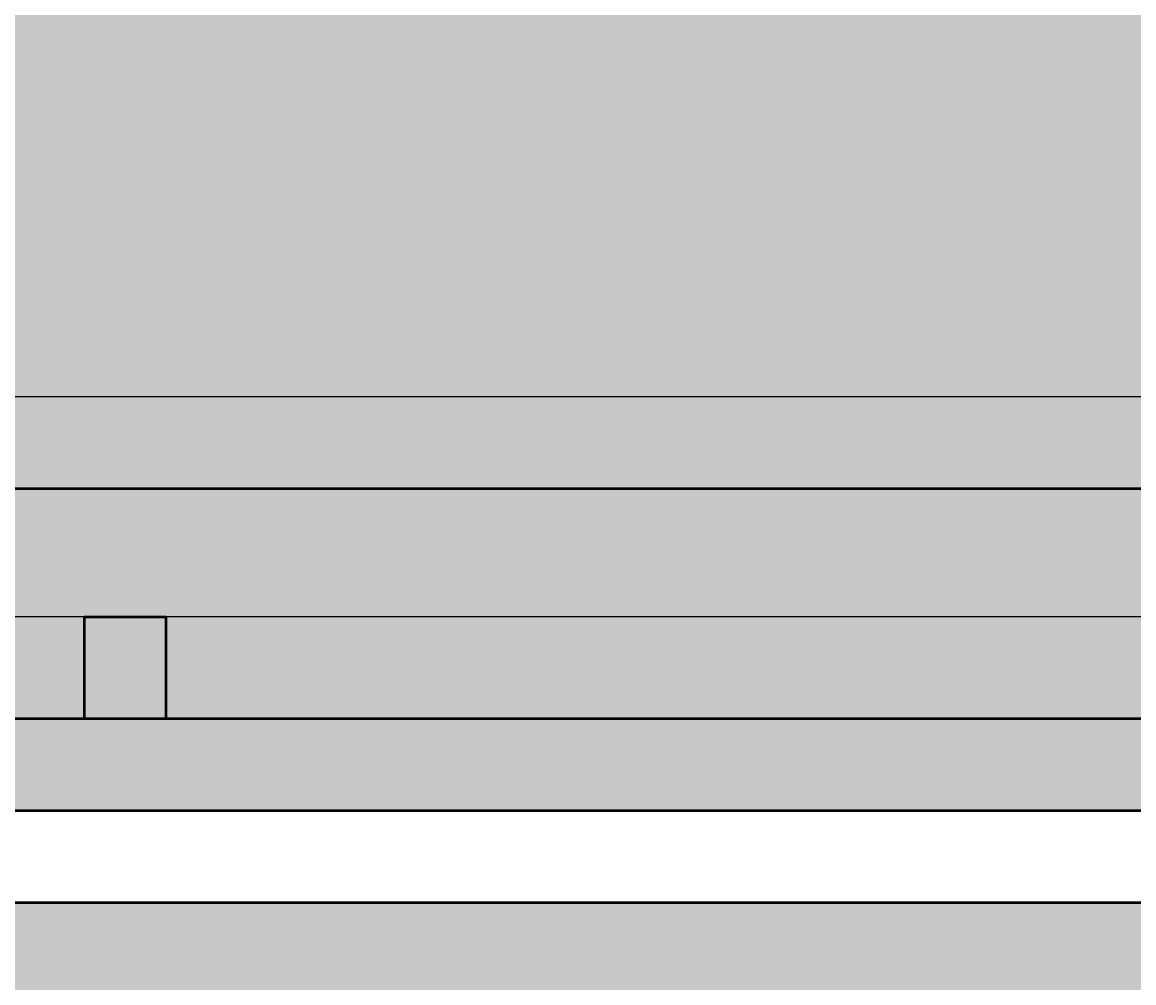
# Model space of a CAD drawing. Units: inches. Extents: x -12 to 334, y -10 to 186.
# Tile 40 of 77: x 128 to 152, y 90 to 111. Entities that reach past the tile are written whole.
import ezdxf
from ezdxf import colors
from ezdxf.entities.mleader import LeaderData, LeaderLine
from ezdxf.math import Vec2, Vec3

# ---------------------------------------------------------------- set-up
doc = ezdxf.new("R2010")
doc.units = ezdxf.units.IN
doc.header["$MEASUREMENT"] = 0
for name, color, linetype, lineweight in [('M-ANNO-TEXT', 3, 'Continuous', 25), ('M-DIMS', 2, 'Continuous', 18), ('M-EQPM', 7, 'Continuous', 50), ('M-EQPM-PATT', 8, 'Continuous', 18)]:
    doc.layers.add(name, color=color, linetype=linetype, lineweight=lineweight)
doc.styles.get("Standard").update_dxf_attribs({"font": 'arial.ttf'})
doc.dimstyles.get("Standard").update_dxf_attribs({"dimtxt": 0.18, "dimasz": 0.18, "dimexe": 0.18, "dimexo": 0.0625, "dimgap": 0.09, "dimtad": 0, "dimtih": 1, "dimtoh": 1, "dimdec": 4, "dimzin": 0, "dimdsep": 46, "dimtxsty": 'Standard', "dimcen": 0.09, "dimadec": 0, "dimazin": 0, "dimtfac": 1, "dimtdec": 4, "dimtofl": 0, "dimtmove": 0, "dimatfit": 3, "dimfxl": 1, "dimtolj": 1, "dimtzin": 0, "dimarcsym": 0})

# ---------------------------------------------------------------- blocks, each defined once
blk = doc.blocks.new('*D1')
at = {"layer": 'Defpoints', "color": 0, "transparency": 16777216}
for p in [(281.426, 91.899), (3.376, 80.692), (281.426, 14.304)]:
    blk.add_point(p, dxfattribs=at)
at = {"layer": 'M-DIMS', "color": 0, "lineweight": -2, "transparency": 16777216}
for p, q in [((281.426, 91.836), (281.426, 14.124)), ((3.376, 80.629), (3.376, 14.124)), ((3.556, 14.304), (141.935, 14.304)), ((281.246, 14.304), (142.867, 14.304))]:
    blk.add_line(p, q, dxfattribs=at)
at = {"layer": 'M-DIMS', "color": 0, "transparency": 16777216}
for points in [[(3.556, 14.334), (3.556, 14.274), (3.376, 14.304)], [(281.246, 14.334), (281.246, 14.274), (281.426, 14.304)]]:
    blk.add_solid(points, dxfattribs=at)
at = {"layer": 'M-DIMS', "color": 0, "transparency": 16777216, "insert": (142.401, 14.304), "char_height": 0.18, "attachment_point": 5}
blk.add_mtext('\\A1;278.05', dxfattribs=at)
blk = doc.blocks.new('*D17')
at = {"layer": 'Defpoints', "color": 0, "transparency": 16777216}
for p in [(106.177, 102.896), (105.892, 56.321), (295.976, 56.321)]:
    blk.add_point(p, dxfattribs=at)
at = {"layer": 'M-DIMS', "color": 0, "lineweight": -2, "transparency": 16777216}
for p, q in [((106.24, 102.896), (296.156, 102.896)), ((295.976, 102.716), (295.976, 79.79)), ((295.976, 56.501), (295.976, 79.426)), ((105.954, 56.321), (296.156, 56.321))]:
    blk.add_line(p, q, dxfattribs=at)
at = {"layer": 'M-DIMS', "color": 0, "transparency": 16777216}
for points in [[(295.946, 102.716), (296.006, 102.716), (295.976, 102.896)], [(295.946, 56.501), (296.006, 56.501), (295.976, 56.321)]]:
    blk.add_solid(points, dxfattribs=at)
at = {"layer": 'M-DIMS', "color": 0, "transparency": 16777216, "insert": (295.976, 79.608), "char_height": 0.18, "attachment_point": 5}
blk.add_mtext('\\A1;46.575', dxfattribs=at)
blk = doc.blocks.new('*D35')
at = {"layer": 'Defpoints', "color": 0, "transparency": 16777216}
for p in [(216.428, 98.108), (-11.174, 61.105), (216.428, 61.105)]:
    blk.add_point(p, dxfattribs=at)
at = {"layer": 'M-DIMS', "color": 0, "lineweight": -2, "transparency": 16777216}
for p, q in [((216.365, 98.108), (-11.354, 98.108)), ((-11.174, 97.928), (-11.174, 79.788)), ((-11.174, 61.285), (-11.174, 79.424)), ((216.365, 61.105), (-11.354, 61.105))]:
    blk.add_line(p, q, dxfattribs=at)
at = {"layer": 'M-DIMS', "color": 0, "transparency": 16777216}
for points in [[(-11.204, 97.928), (-11.144, 97.928), (-11.174, 98.108)], [(-11.204, 61.285), (-11.144, 61.285), (-11.174, 61.105)]]:
    blk.add_solid(points, dxfattribs=at)
at = {"layer": 'M-DIMS', "color": 0, "transparency": 16777216, "insert": (-11.174, 79.606), "char_height": 0.18, "attachment_point": 5}
blk.add_mtext('\\A1;37', dxfattribs=at)

msp = doc.modelspace()

# ---------------------------------------------------------------- hatches: boundary and pattern name
at = {"layer": 'M-EQPM-PATT', "transparency": 33554556}
h = msp.add_hatch(color=256, dxfattribs=at)
h.set_gradient(color1=(248, 206, 179), color2=(248, 206, 179), tint=1)
h.paths.add_polyline_path([(179.7818, 136.8871), (126.9567, 136.8871), (106.1771, 100.8958), (171.5458, 100.8958)])
h.paths.add_polyline_path([(268.3808, 136.9435), (214.0166, 136.9435), (214.0166, 154.8345), (196.3421, 154.8345), (196.3421, 136.8871), (179.7818, 136.8871), (171.5458, 100.8958), (231.7758, 100.8958, -0.4142136), (251.9801, 80.6915), (279.7263, 80.6915, 0.1631825)])
at = {"layer": 'M-EQPM-PATT'}
h = msp.add_hatch(color=256, dxfattribs=at)
h.set_gradient(color1=(205, 32, 39), color2=(205, 32, 39), tint=1)
h.paths.add_polyline_path([(64.5, 80.754), (64.5, 89.8963), (226.6083, 89.8963, -1), (226.6083, 69.6117), (64.5, 69.6117), (64.5, 78.754), (4.4744, 78.754, 0.384914), (23.5807, 61.4872), (37.1002, 61.4872), (37.1002, 33.6752), (53.1002, 33.6752), (53.1002, 61.4872), (64.5, 61.4872), (64.5, 63.6117), (226.6083, 63.6117, 1), (226.6083, 95.8963), (64.5, 95.8963), (64.5, 99.8958), (53.1002, 99.8958), (53.1002, 127.7078), (37.1002, 127.7078), (37.1002, 99.8958), (23.5807, 99.8958, 0.4132606), (4.3766, 80.754)])
h.paths.add_polyline_path([(64.5, 91.8963), (64.5, 93.8963), (226.6083, 93.8963, -1), (226.6083, 65.6117), (64.5, 65.6117), (64.5, 67.6117), (226.6083, 67.6117, 1), (226.6083, 91.8963)], flags=16)
h = msp.add_hatch(color=256, dxfattribs=at)
h.set_gradient(color1=(99, 100, 102), color2=(99, 100, 102), tint=1)
h.paths.add_polyline_path([(72.9244, 95.8963), (75.9244, 95.8963), (75.9244, 109.0583), (72.9244, 109.0583)])
h.paths.add_polyline_path([(72.9244, 50.4497), (75.9244, 50.4497), (75.9244, 63.6117), (72.9244, 63.6117)])
h.paths.add_polyline_path([(75.9244, 91.8963), (75.9244, 93.8963), (72.9244, 93.8963), (72.9244, 91.8963)])
h.paths.add_polyline_path([(75.9244, 65.6117), (75.9244, 67.6117), (72.9244, 67.6117), (72.9244, 65.6117)])
h.paths.add_polyline_path([(129.093, 69.6117), (130.8573, 69.6117), (130.8573, 89.8963), (129.093, 89.8963)])
h.paths.add_polyline_path([(129.093, 98.1081), (129.093, 95.8963), (130.8573, 95.8963), (130.8573, 98.1081)])
h.paths.add_polyline_path([(130.8573, 61.1045), (130.8573, 63.6117), (129.093, 63.6117), (129.093, 61.1045)])
h.paths.add_polyline_path([(170.9079, 69.6117), (172.6722, 69.6117), (172.6722, 89.8963), (170.9079, 89.8963)])
h.paths.add_polyline_path([(172.6722, 95.8963), (172.6722, 98.1081), (170.9079, 98.1081), (170.9079, 95.8963)])
h.paths.add_polyline_path([(170.9079, 61.1045), (172.6722, 61.1045), (172.6722, 63.6117), (170.9079, 63.6117)])
h.paths.add_polyline_path([(218.1922, 63.6117), (216.4278, 63.6117), (216.4278, 61.1045), (218.1922, 61.1045)])
h.paths.add_polyline_path([(216.4278, 69.6117), (218.1922, 69.6117), (218.1922, 89.8963), (216.4278, 89.8963)])
h.paths.add_polyline_path([(216.4278, 95.8963), (218.1922, 95.8963), (218.1922, 98.1081), (216.4278, 98.1081)])
h = msp.add_hatch(color=256, dxfattribs=at)
h.set_gradient(color1=(94, 103, 175), color2=(94, 103, 175), tint=1)
h.paths.add_polyline_path([(129.093, 89.8963), (86.8879, 89.8963), (86.8879, 69.6117), (129.093, 69.6117)], flags=17)
h.paths.add_polyline_path([(170.9079, 89.8963), (130.8573, 89.8963), (130.8573, 69.6117), (170.9079, 69.6117)], flags=17)
h.paths.add_polyline_path([(216.4278, 89.8963), (172.6722, 89.8963), (172.6722, 69.6117), (216.4278, 69.6117)], flags=17)
h.paths.add_polyline_path([(245.9354, 82.6969), (247.9354, 82.6969), (247.9354, 46.8541), (268.3808, 46.8541, 0.0998398), (279.7263, 80.6915), (251.9801, 80.6915, 0.4142136), (231.7758, 100.8958), (84.7229, 100.8958), (84.7229, 109.0583), (83.7229, 109.0583), (83.7229, 95.8963), (129.093, 95.8963), (129.093, 98.1081), (130.8573, 98.1081), (130.8573, 95.8963), (170.9079, 95.8963), (170.9079, 98.1081), (172.6722, 98.1081), (172.6722, 95.8963), (216.4278, 95.8963), (216.4278, 98.1081), (218.1922, 98.1081), (218.1922, 95.8963), (226.6083, 95.8963, -1), (226.6083, 63.6117), (218.1922, 63.6117), (218.1922, 61.1045), (216.4278, 61.1045), (216.4278, 63.6117), (172.6722, 63.6117), (172.6722, 61.1045), (170.9079, 61.1045), (170.9079, 63.6117), (130.8573, 63.6117), (130.8573, 61.1045), (129.093, 61.1045), (129.093, 63.6117), (87.8879, 63.6117), (87.8879, 56.3205), (105.8919, 56.3205), (105.8919, 28.8541), (115.8919, 28.8541), (115.8919, 46.8541), (222.5761, 46.8541), (222.5761, 30.8541), (232.5761, 30.8541), (232.5761, 46.8541), (245.9354, 46.8541)])
h.paths.add_polyline_path([(86.8879, 89.8963), (75.9244, 89.8963), (75.9244, 69.6117), (86.8879, 69.6117)])
h.paths.add_polyline_path([(83.7229, 109.0583), (75.9244, 109.0583), (75.9244, 95.8963), (83.7229, 95.8963)])
h.paths.add_polyline_path([(226.6083, 89.8963), (218.1922, 89.8963), (218.1922, 69.6117), (226.6083, 69.6117, 1)], flags=17)
h = msp.add_hatch(color=256, dxfattribs=at)
h.set_gradient(color1=(0, 0, 255), color2=(0, 0, 255), tint=1)
h.paths.add_polyline_path([(84.7229, 100.8958), (84.7229, 109.0583), (83.7229, 109.0583), (83.7229, 95.8963), (129.093, 95.8963), (129.093, 98.1081), (130.8573, 98.1081), (130.8573, 95.8963), (170.9079, 95.8963), (170.9079, 98.1081), (172.6722, 98.1081), (172.6722, 95.8963), (216.4278, 95.8963), (216.4278, 98.1081), (218.1922, 98.1081), (218.1922, 95.8963), (226.6083, 95.8963, -1), (226.6083, 63.6117), (218.1922, 63.6117), (218.1922, 61.1045), (216.4278, 61.1045), (216.4278, 63.6117), (172.6722, 63.6117), (172.6722, 61.1045), (170.9079, 61.1045), (170.9079, 63.6117), (130.8573, 63.6117), (130.8573, 61.1045), (129.093, 61.1045), (129.093, 63.6117), (87.8879, 63.6117), (87.8879, 56.3205), (105.8919, 56.3205), (105.8919, 28.8541), (115.8919, 28.8541), (115.8919, 46.8541), (222.5761, 46.8541), (222.5761, 30.8541), (232.5761, 30.8541), (232.5761, 46.8541), (245.9354, 46.8541), (245.9354, 82.6969), (247.9354, 82.6969), (247.9354, 46.8541), (268.3808, 46.8541, 0.0998398), (279.7263, 80.6915), (251.9801, 80.6915, 0.4142136), (231.7758, 100.8958)])

# ---------------------------------------------------------------- linework, layer by layer
at = {"layer": 'M-EQPM'}
for points in [[(84.7229, 100.8958), (231.7758, 100.8958)], [(129.093, 95.8963), (129.093, 98.1081), (130.8573, 98.1081), (130.8573, 95.8963)]]:
    msp.add_lwpolyline(points, dxfattribs=at)
for points in [[(64.5, 63.6117), (226.6083, 63.6117, 1), (226.6083, 95.8963), (64.5, 95.8963)], [(64.5, 65.6117), (226.6083, 65.6117, 1), (226.6083, 93.8963), (64.5, 93.8963)], [(64.5, 67.6117), (226.6083, 67.6117, 1), (226.6083, 91.8963), (64.5, 91.8963)]]:
    msp.add_lwpolyline(points, format="xyb", dxfattribs=at)

# ---------------------------------------------------------------- dimensions: what is measured, and where the dimension line sits
at = {"layer": 'M-DIMS'}
for base, p1, p2, override, picture, middle in [((295.9756, 56.3205), (106.1771, 102.8958), (105.8919, 56.3205), {"dimdec": 3, "dimlfac": 1, "dimrnd": 0, "dimzin": 0, "dimdsep": 46, "dimlunit": 2}, '*D17', (295.9756, 79.6082)), ((-11.1736, 61.1045), (216.4278, 98.1081), (216.4278, 61.1045), {"dimdec": 0, "dimlfac": 1, "dimrnd": 0, "dimzin": 0, "dimdsep": 46, "dimlunit": 2}, '*D35', (-11.1735, 79.6063))]:
    dim = msp.add_linear_dim(base=base, p1=p1, p2=p2, angle=90, dimstyle='Standard', override=override, dxfattribs=at)
    dim.commit()
    dim.dimension.update_dxf_attribs({"geometry": picture, "text_midpoint": middle})
dim = msp.add_linear_dim(base=(281.4256, 14.3041), p1=(3.3765, 80.6915), p2=(281.4256, 91.8988), dimstyle='Standard', override={"dimdec": 2, "dimlfac": 1, "dimrnd": 0, "dimzin": 0, "dimdsep": 46, "dimlunit": 2}, dxfattribs=at)
dim.commit()
dim.dimension.update_dxf_attribs({"geometry": '*D1', "text_midpoint": (142.401, 14.3041)})

# ---------------------------------------------------------------- leaders
at = {"layer": 'M-ANNO-TEXT'}
ml = msp.add_multileader_mtext('Standard', dxfattribs=at)
ml.set_content('Tube supports', color=256)
ml.set_leader_properties()
ml.build(insert=Vec2(0, 0))
ml.multileader.update_dxf_attribs({"dogleg_length": 0.36, "arrow_head_size": 0.7})
ctx = ml.context
ctx.base_point, ctx.arrow_head_size, ctx.landing_gap_size, ctx.plane_origin = Vec3(129.4363, 148.4609), 0.7, 0.09, Vec3(117.375, 151.6517)
ctx.text_align_type = 2
notes = []
notes.append((ctx, [(1, (1, 1, 0), (182.4302, 148.4609), (-1, 0), 17.4388, [(0, [(170.9079, 98.1081)], 0, [])])]))
ctx.mtext.insert, ctx.mtext.alignment, ctx.mtext.flow_direction = Vec3(164.9015, 151.0162), 3, 5
for ctx, leaders in notes:
    for number, flags, end, landing, length, lines in leaders:
        leader = LeaderData()
        leader.index, (leader.has_last_leader_line, leader.has_dogleg_vector, leader.attachment_direction) = number, flags
        leader.last_leader_point, leader.dogleg_vector, leader.dogleg_length = Vec3(end), Vec3(landing), length
        for number, points, colour, breaks in lines:
            line = LeaderLine()
            line.index, line.vertices, line.color, line.breaks = number, Vec3.list(points), colors.encode_raw_color(colour), breaks
            leader.lines.append(line)
        ctx.leaders.append(leader)

doc.saveas('drawing.dxf')
